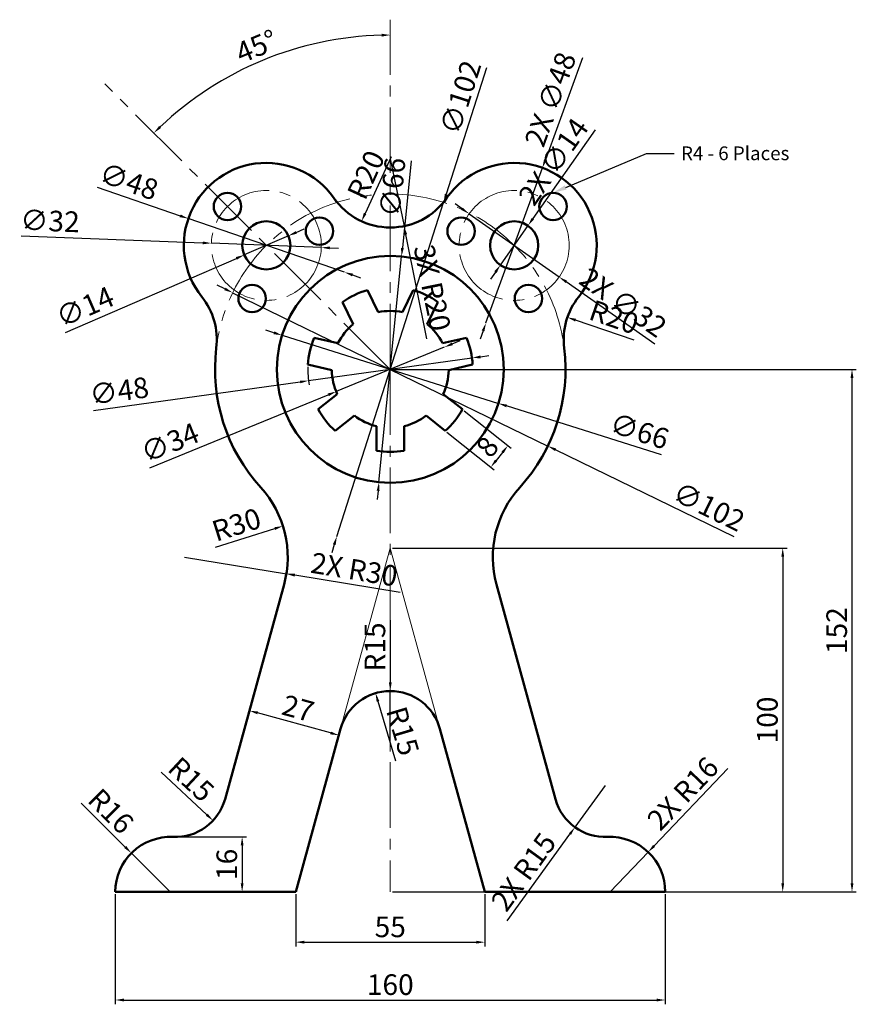
# Model space of a CAD drawing. Units: millimetres. Extents: x 3162 to 3406, y 1893 to 2179.
import ezdxf
from ezdxf import colors
from ezdxf.entities.mleader import LeaderData, LeaderLine
from ezdxf.math import Vec2, Vec3

# ---------------------------------------------------------------- set-up
doc = ezdxf.new("R2010")
doc.units = ezdxf.units.MM
doc.linetypes.add('CENTER2', pattern=[28.575, 19.05, -3.175, 3.175, -3.175])
for name, color, linetype, lineweight in [('M-CNTR', 51, 'CENTER2', 18), ('M-CONS', 8, 'Continuous', 13), ('M-DIMS', 2, 'Continuous', 25), ('M-OUTL', 7, 'Continuous', 50), ('M-TEXT', 7, 'Continuous', 25)]:
    doc.layers.add(name, color=color, linetype=linetype, lineweight=lineweight)
doc.styles.get("Standard").update_dxf_attribs({"font": 'arial.ttf'})
doc.dimstyles.new('ISO-25', dxfattribs={"dimtxt": 6, "dimasz": 2.5, "dimexe": 1.25, "dimexo": 0.625, "dimtad": 1, "dimtxsty": 'Standard', "dimcen": 2.5, "dimadec": 0, "dimazin": 0, "dimtfac": 1, "dimtmove": 0, "dimatfit": 3, "dimfxl": 1, "dimarcsym": 0})

# ---------------------------------------------------------------- blocks, each defined once
blk = doc.blocks.new('*D1')
at = {"layer": 'Defpoints', "color": 0, "transparency": 16777216}
for p in [(3242.62, 1925.58), (3297.62, 1925.58), (3297.62, 1910.95)]:
    blk.add_point(p, dxfattribs=at)
at = {"layer": 'M-DIMS', "color": 0, "lineweight": -2, "transparency": 16777216}
for p, q in [((3242.62, 1924.95), (3242.62, 1909.7)), ((3297.62, 1924.95), (3297.62, 1909.7)), ((3245.12, 1910.95), (3295.12, 1910.95))]:
    blk.add_line(p, q, dxfattribs=at)
at = {"layer": 'M-DIMS', "color": 0, "transparency": 16777216}
for points in [[(3245.12, 1911.37), (3245.12, 1910.53), (3242.62, 1910.95)], [(3295.12, 1911.37), (3295.12, 1910.53), (3297.62, 1910.95)]]:
    blk.add_solid(points, dxfattribs=at)
at = {"layer": 'M-DIMS', "color": 0, "transparency": 16777216, "insert": (3270.12, 1914.63), "char_height": 6, "attachment_point": 5}
blk.add_mtext('55', dxfattribs=at)
blk = doc.blocks.new('*D2')
at = {"layer": 'Defpoints', "color": 0, "transparency": 16777216}
for p in [(3190.12, 1925.58), (3350.12, 1925.58), (3350.12, 1894.13)]:
    blk.add_point(p, dxfattribs=at)
at = {"layer": 'M-DIMS', "color": 0, "lineweight": -2, "transparency": 16777216}
for p, q in [((3190.12, 1924.95), (3190.12, 1892.88)), ((3350.12, 1924.95), (3350.12, 1892.88)), ((3192.62, 1894.13), (3347.62, 1894.13))]:
    blk.add_line(p, q, dxfattribs=at)
at = {"layer": 'M-DIMS', "color": 0, "transparency": 16777216}
for points in [[(3192.62, 1894.54), (3192.62, 1893.71), (3190.12, 1894.13)], [(3347.62, 1894.54), (3347.62, 1893.71), (3350.12, 1894.13)]]:
    blk.add_solid(points, dxfattribs=at)
at = {"layer": 'M-DIMS', "color": 0, "transparency": 16777216, "insert": (3270.12, 1897.82), "char_height": 6, "attachment_point": 5}
blk.add_mtext('160', dxfattribs=at)
blk = doc.blocks.new('*D3')
at = {"layer": 'Defpoints', "color": 0, "transparency": 16777216}
for p in [(3270.12, 2025.58), (3270.12, 1925.58), (3384.31, 1925.58)]:
    blk.add_point(p, dxfattribs=at)
at = {"layer": 'M-DIMS', "color": 0, "lineweight": -2, "transparency": 16777216}
for p, q in [((3270.74, 2025.58), (3385.56, 2025.58)), ((3384.31, 2023.08), (3384.31, 1928.08)), ((3270.74, 1925.58), (3385.56, 1925.58))]:
    blk.add_line(p, q, dxfattribs=at)
at = {"layer": 'M-DIMS', "color": 0, "transparency": 16777216}
for points in [[(3383.9, 2023.08), (3384.73, 2023.08), (3384.31, 2025.58)], [(3383.9, 1928.08), (3384.73, 1928.08), (3384.31, 1925.58)]]:
    blk.add_solid(points, dxfattribs=at)
at = {"layer": 'M-DIMS', "color": 0, "transparency": 16777216, "insert": (3380.62, 1975.58), "char_height": 6, "attachment_point": 5, "rotation": 90}
blk.add_mtext('100', dxfattribs=at)
blk = doc.blocks.new('*D4')
at = {"layer": 'Defpoints', "color": 0, "transparency": 16777216}
for p in [(3270.12, 2077.58), (3404.47, 2077.58), (3270.12, 1925.58)]:
    blk.add_point(p, dxfattribs=at)
at = {"layer": 'M-DIMS', "color": 0, "lineweight": -2, "transparency": 16777216}
for p, q in [((3270.74, 2077.58), (3405.72, 2077.58)), ((3404.47, 1928.08), (3404.47, 2075.08)), ((3270.74, 1925.58), (3405.72, 1925.58))]:
    blk.add_line(p, q, dxfattribs=at)
at = {"layer": 'M-DIMS', "color": 0, "transparency": 16777216}
for points in [[(3404.06, 2075.08), (3404.89, 2075.08), (3404.47, 2077.58)], [(3404.06, 1928.08), (3404.89, 1928.08), (3404.47, 1925.58)]]:
    blk.add_solid(points, dxfattribs=at)
at = {"layer": 'M-DIMS', "color": 0, "transparency": 16777216, "insert": (3400.79, 2001.58), "char_height": 6, "attachment_point": 5, "rotation": 90}
blk.add_mtext('152', dxfattribs=at)
blk = doc.blocks.new('*D5')
at = {"layer": 'Defpoints', "color": 0, "transparency": 16777216}
for p in [(3206.12, 1941.58), (3206.12, 1925.58), (3227.02, 1925.58)]:
    blk.add_point(p, dxfattribs=at)
at = {"layer": 'M-DIMS', "color": 0, "lineweight": -2, "transparency": 16777216}
for p, q in [((3206.74, 1941.58), (3228.27, 1941.58)), ((3227.02, 1939.08), (3227.02, 1928.08)), ((3206.74, 1925.58), (3228.27, 1925.58))]:
    blk.add_line(p, q, dxfattribs=at)
at = {"layer": 'M-DIMS', "color": 0, "transparency": 16777216}
for points in [[(3226.6, 1939.08), (3227.44, 1939.08), (3227.02, 1941.58)], [(3226.6, 1928.08), (3227.44, 1928.08), (3227.02, 1925.58)]]:
    blk.add_solid(points, dxfattribs=at)
at = {"layer": 'M-DIMS', "color": 0, "transparency": 16777216, "insert": (3223.33, 1933.58), "char_height": 6, "attachment_point": 5, "rotation": 90}
blk.add_mtext('16', dxfattribs=at)
blk = doc.blocks.new('*D6')
at = {"layer": 'Defpoints', "color": 0, "transparency": 16777216}
for p in [(3229.62, 1980.15), (3229.12, 1978.3), (3255.66, 1972.99)]:
    blk.add_point(p, dxfattribs=at)
at = {"layer": 'M-DIMS', "color": 0, "lineweight": -2, "transparency": 16777216}
for p, q in [((3229.46, 1979.54), (3228.78, 1977.1)), ((3252.74, 1971.81), (3231.53, 1977.64)), ((3255.49, 1972.38), (3254.82, 1969.94))]:
    blk.add_line(p, q, dxfattribs=at)
at = {"layer": 'M-DIMS', "color": 0, "transparency": 16777216}
for points in [[(3231.64, 1978.04), (3231.42, 1977.24), (3229.12, 1978.3)], [(3252.85, 1972.21), (3252.63, 1971.41), (3255.15, 1971.15)]]:
    blk.add_solid(points, dxfattribs=at)
at = {"layer": 'M-DIMS', "color": 0, "transparency": 16777216, "insert": (3243.1, 1978.23), "char_height": 6, "attachment_point": 5, "rotation": 344.6237}
blk.add_mtext('27', dxfattribs=at)
blk = doc.blocks.new('*D7')
at = {"layer": 'Defpoints', "color": 0, "transparency": 16777216}
for p in [(3194.78, 1936.87), (3206.12, 1925.58)]:
    blk.add_point(p, dxfattribs=at)
at = {"layer": 'M-DIMS', "color": 0, "lineweight": -2, "transparency": 16777216}
for p, q in [((3180.2, 1951.39), (3193.01, 1938.63)), ((3206.12, 1925.58), (3194.78, 1936.87))]:
    blk.add_line(p, q, dxfattribs=at)
at = {"layer": 'M-DIMS', "color": 0, "transparency": 16777216}
blk.add_solid([(3193.3, 1938.93), (3192.72, 1938.34), (3194.78, 1936.87)], dxfattribs=at)
at = {"layer": 'M-DIMS', "color": 0, "transparency": 16777216, "insert": (3188.32, 1948.51), "char_height": 6, "attachment_point": 5, "rotation": 315.1198}
blk.add_mtext('R16', dxfattribs=at)
blk = doc.blocks.new('*D8')
at = {"layer": 'Defpoints', "color": 0, "transparency": 16777216}
for p in [(3207.57, 1956.55), (3218.55, 1946.33)]:
    blk.add_point(p, dxfattribs=at)
at = {"layer": 'M-DIMS', "color": 0, "lineweight": -2, "transparency": 16777216}
blk.add_line((3203.45, 1960.38), (3216.72, 1948.03), dxfattribs=at)
at = {"layer": 'M-DIMS', "color": 0, "transparency": 16777216}
blk.add_solid([(3217.01, 1948.33), (3216.44, 1947.72), (3218.55, 1946.33)], dxfattribs=at)
at = {"layer": 'M-DIMS', "color": 0, "transparency": 16777216, "insert": (3211.69, 1957.76), "char_height": 6, "attachment_point": 5, "rotation": 317.0538}
blk.add_mtext('R15', dxfattribs=at)
blk = doc.blocks.new('*D9')
at = {"layer": 'Defpoints', "color": 0, "transparency": 16777216}
for p in [(3265.84, 1983.39), (3270.12, 1969.01)]:
    blk.add_point(p, dxfattribs=at)
at = {"layer": 'M-DIMS', "color": 0, "lineweight": -2, "transparency": 16777216}
blk.add_line((3271.73, 1963.61), (3266.55, 1980.99), dxfattribs=at)
at = {"layer": 'M-DIMS', "color": 0, "transparency": 16777216}
blk.add_solid([(3266.95, 1981.11), (3266.15, 1980.87), (3265.84, 1983.39)], dxfattribs=at)
at = {"layer": 'M-DIMS', "color": 0, "transparency": 16777216, "insert": (3273.03, 1972.15), "char_height": 6, "attachment_point": 5, "rotation": 286.5756}
blk.add_mtext('R15', dxfattribs=at)
blk = doc.blocks.new('*D10')
at = {"layer": 'Defpoints', "color": 0, "transparency": 16777216}
for p in [(3238.9, 2032), (3210.29, 2022.98)]:
    blk.add_point(p, dxfattribs=at)
at = {"layer": 'M-DIMS', "color": 0, "lineweight": -2, "transparency": 16777216}
blk.add_line((3219.28, 2025.82), (3236.51, 2031.25), dxfattribs=at)
at = {"layer": 'M-DIMS', "color": 0, "transparency": 16777216}
blk.add_solid([(3236.39, 2031.65), (3236.64, 2030.86), (3238.9, 2032)], dxfattribs=at)
at = {"layer": 'M-DIMS', "color": 0, "transparency": 16777216, "insert": (3225.6, 2031.68), "char_height": 6, "attachment_point": 5, "rotation": 17.5099}
blk.add_mtext('R30', dxfattribs=at)
blk = doc.blocks.new('*D11')
at = {"layer": 'Defpoints', "color": 0, "transparency": 16777216}
for p in [(3291.11, 2065.95), (3286.13, 2059.7), (3299.37, 2049.14)]:
    blk.add_point(p, dxfattribs=at)
at = {"layer": 'M-DIMS', "color": 0, "lineweight": -2, "transparency": 16777216}
for p, q in [((3291.6, 2065.56), (3305.33, 2054.61)), ((3286.61, 2059.31), (3300.35, 2048.36)), ((3302.8, 2053.44), (3300.93, 2051.09))]:
    blk.add_line(p, q, dxfattribs=at)
at = {"layer": 'M-DIMS', "color": 0, "transparency": 16777216}
for points in [[(3302.47, 2053.7), (3303.12, 2053.18), (3304.36, 2055.39)], [(3300.6, 2051.35), (3301.25, 2050.83), (3299.37, 2049.14)]]:
    blk.add_solid(points, dxfattribs=at)
at = {"layer": 'M-DIMS', "color": 0, "transparency": 16777216, "insert": (3298.98, 2054.56), "char_height": 6, "attachment_point": 5, "rotation": 51.4286}
blk.add_mtext('8', dxfattribs=at)
blk = doc.blocks.new('*D12')
at = {"layer": 'Defpoints', "color": 0, "transparency": 16777216}
for p in [(3321.67, 2092.7), (3340.59, 2086.22)]:
    blk.add_point(p, dxfattribs=at)
at = {"layer": 'M-DIMS', "color": 0, "lineweight": -2, "transparency": 16777216}
blk.add_line((3341.13, 2086.04), (3324.04, 2091.89), dxfattribs=at)
at = {"layer": 'M-DIMS', "color": 0, "transparency": 16777216}
blk.add_solid([(3324.17, 2092.29), (3323.9, 2091.5), (3321.67, 2092.7)], dxfattribs=at)
at = {"layer": 'M-DIMS', "color": 0, "transparency": 16777216, "insert": (3334.96, 2092.05), "char_height": 6, "attachment_point": 5, "rotation": 341.084}
blk.add_mtext('R20', dxfattribs=at)
blk = doc.blocks.new('*D13')
at = {"layer": 'Defpoints', "color": 0, "transparency": 16777216}
for p in [(3270.12, 2138.85), (3261.77, 2120.68)]:
    blk.add_point(p, dxfattribs=at)
at = {"layer": 'M-DIMS', "color": 0, "lineweight": -2, "transparency": 16777216}
blk.add_line((3270.36, 2139.37), (3262.81, 2122.95), dxfattribs=at)
at = {"layer": 'M-DIMS', "color": 0, "transparency": 16777216}
blk.add_solid([(3262.43, 2123.12), (3263.19, 2122.78), (3261.77, 2120.68)], dxfattribs=at)
at = {"layer": 'M-DIMS', "color": 0, "transparency": 16777216, "insert": (3263.75, 2133.83), "char_height": 6, "attachment_point": 5, "rotation": 65.316}
blk.add_mtext('R20', dxfattribs=at)
blk = doc.blocks.new('*D14')
at = {"layer": 'Defpoints', "color": 0, "transparency": 16777216}
for p in [(3211.35, 2121.43), (3256.76, 2105.85)]:
    blk.add_point(p, dxfattribs=at)
at = {"layer": 'M-DIMS', "color": 0, "lineweight": -2, "transparency": 16777216}
for p, q in [((3184.81, 2130.54), (3208.99, 2122.24)), ((3256.76, 2105.85), (3211.35, 2121.43)), ((3259.12, 2105.04), (3261.49, 2104.23))]:
    blk.add_line(p, q, dxfattribs=at)
at = {"layer": 'M-DIMS', "color": 0, "transparency": 16777216}
for points in [[(3209.13, 2122.63), (3208.85, 2121.85), (3211.35, 2121.43)], [(3259.26, 2105.44), (3258.99, 2104.65), (3256.76, 2105.85)]]:
    blk.add_solid(points, dxfattribs=at)
at = {"layer": 'M-DIMS', "color": 0, "transparency": 16777216, "insert": (3193.81, 2131.52), "char_height": 6, "attachment_point": 5, "rotation": 341.0657}
blk.add_mtext('∅48', dxfattribs=at)
blk = doc.blocks.new('*D15')
at = {"layer": 'Defpoints', "color": 0, "transparency": 16777216}
for p in [(3218.07, 2114.28), (3250.04, 2113.01)]:
    blk.add_point(p, dxfattribs=at)
at = {"layer": 'M-DIMS', "color": 0, "lineweight": -2, "transparency": 16777216}
for p, q in [((3162.77, 2116.47), (3215.57, 2114.38)), ((3250.04, 2113.01), (3218.07, 2114.28)), ((3252.54, 2112.91), (3255.04, 2112.81))]:
    blk.add_line(p, q, dxfattribs=at)
at = {"layer": 'M-DIMS', "color": 0, "transparency": 16777216}
for points in [[(3215.59, 2114.79), (3215.55, 2113.96), (3218.07, 2114.28)], [(3252.56, 2113.32), (3252.52, 2112.49), (3250.04, 2113.01)]]:
    blk.add_solid(points, dxfattribs=at)
at = {"layer": 'M-DIMS', "color": 0, "transparency": 16777216, "insert": (3171.08, 2120), "char_height": 6, "attachment_point": 5, "rotation": 357.726}
blk.add_mtext('∅32', dxfattribs=at)
blk = doc.blocks.new('*D16')
at = {"layer": 'Defpoints', "color": 0, "transparency": 16777216}
for p in [(3240.48, 2116.43), (3227.63, 2110.86)]:
    blk.add_point(p, dxfattribs=at)
at = {"layer": 'M-DIMS', "color": 0, "lineweight": -2, "transparency": 16777216}
for p, q in [((3242.77, 2117.42), (3245.06, 2118.42)), ((3240.48, 2116.43), (3227.63, 2110.86)), ((3175.62, 2088.29), (3225.34, 2109.86))]:
    blk.add_line(p, q, dxfattribs=at)
at = {"layer": 'M-DIMS', "color": 0, "transparency": 16777216}
for points in [[(3242.61, 2117.81), (3242.94, 2117.04), (3240.48, 2116.43)], [(3225.18, 2110.24), (3225.51, 2109.48), (3227.63, 2110.86)]]:
    blk.add_solid(points, dxfattribs=at)
at = {"layer": 'M-DIMS', "color": 0, "transparency": 16777216, "insert": (3181.59, 2095.08), "char_height": 6, "attachment_point": 5, "rotation": 23.4555}
blk.add_mtext('∅14', dxfattribs=at)
blk = doc.blocks.new('*D17')
at = {"layer": 'Defpoints', "color": 0, "transparency": 16777216}
for p in [(3293.89, 2080.88), (3246.35, 2074.28)]:
    blk.add_point(p, dxfattribs=at)
at = {"layer": 'M-DIMS', "color": 0, "lineweight": -2, "transparency": 16777216}
for p, q in [((3293.89, 2080.88), (3246.35, 2074.28)), ((3296.37, 2081.23), (3298.84, 2081.57)), ((3183.75, 2065.58), (3243.87, 2073.93))]:
    blk.add_line(p, q, dxfattribs=at)
blk.add_arc((3270.12, 2077.58), 24, 178.229, 190.8951, dxfattribs=at)
at = {"layer": 'M-DIMS', "color": 0, "transparency": 16777216}
for points in [[(3296.31, 2081.64), (3296.42, 2080.81), (3293.89, 2080.88)], [(3243.81, 2074.34), (3243.93, 2073.52), (3246.35, 2074.28)]]:
    blk.add_solid(points, dxfattribs=at)
at = {"layer": 'M-DIMS', "color": 0, "transparency": 16777216, "insert": (3191.34, 2070.53), "char_height": 6, "attachment_point": 5, "rotation": 7.9109}
blk.add_mtext('∅48', dxfattribs=at)
blk = doc.blocks.new('*D18')
at = {"layer": 'Defpoints', "color": 0, "transparency": 16777216}
for p in [(3285.85, 2084.03), (3254.39, 2071.13)]:
    blk.add_point(p, dxfattribs=at)
at = {"layer": 'M-DIMS', "color": 0, "lineweight": -2, "transparency": 16777216}
for p, q in [((3288.16, 2084.98), (3290.47, 2085.93)), ((3285.85, 2084.03), (3254.39, 2071.13)), ((3200.19, 2048.89), (3252.08, 2070.18))]:
    blk.add_line(p, q, dxfattribs=at)
at = {"layer": 'M-DIMS', "color": 0, "transparency": 16777216}
for points in [[(3288, 2085.37), (3288.32, 2084.6), (3285.85, 2084.03)], [(3251.92, 2070.56), (3252.24, 2069.79), (3254.39, 2071.13)]]:
    blk.add_solid(points, dxfattribs=at)
at = {"layer": 'M-DIMS', "color": 0, "transparency": 16777216, "insert": (3206.29, 2055.56), "char_height": 6, "attachment_point": 5, "rotation": 22.3094}
blk.add_mtext('∅34', dxfattribs=at)
blk = doc.blocks.new('*D19')
at = {"layer": 'Defpoints', "color": 0, "transparency": 16777216}
for p in [(3238.64, 2087.48), (3301.6, 2067.68)]:
    blk.add_point(p, dxfattribs=at)
at = {"layer": 'M-DIMS', "color": 0, "lineweight": -2, "transparency": 16777216}
for p, q in [((3236.25, 2088.23), (3233.87, 2088.98)), ((3238.64, 2087.48), (3301.6, 2067.68)), ((3349.05, 2052.75), (3303.98, 2066.93))]:
    blk.add_line(p, q, dxfattribs=at)
at = {"layer": 'M-DIMS', "color": 0, "transparency": 16777216}
for points in [[(3236.38, 2088.63), (3236.13, 2087.83), (3238.64, 2087.48)], [(3304.11, 2067.33), (3303.86, 2066.53), (3301.6, 2067.68)]]:
    blk.add_solid(points, dxfattribs=at)
at = {"layer": 'M-DIMS', "color": 0, "transparency": 16777216, "insert": (3342.4, 2058.89), "char_height": 6, "attachment_point": 5, "rotation": 342.54}
blk.add_mtext('∅66', dxfattribs=at)
blk = doc.blocks.new('*D20')
at = {"layer": 'Defpoints', "color": 0, "transparency": 16777216}
for p in [(3224.26, 2099.88), (3315.98, 2055.27)]:
    blk.add_point(p, dxfattribs=at)
at = {"layer": 'M-DIMS', "color": 0, "lineweight": -2, "transparency": 16777216}
for p, q in [((3222.01, 2100.98), (3219.76, 2102.07)), ((3224.26, 2099.88), (3315.98, 2055.27)), ((3370.23, 2028.89), (3318.23, 2054.18))]:
    blk.add_line(p, q, dxfattribs=at)
at = {"layer": 'M-DIMS', "color": 0, "transparency": 16777216}
for points in [[(3222.19, 2101.35), (3221.82, 2100.6), (3224.26, 2099.88)], [(3318.41, 2054.55), (3318.05, 2053.81), (3315.98, 2055.27)]]:
    blk.add_solid(points, dxfattribs=at)
at = {"layer": 'M-DIMS', "color": 0, "transparency": 16777216, "insert": (3362.49, 2036.95), "char_height": 6, "attachment_point": 5, "rotation": 334.0641}
blk.add_mtext('∅102', dxfattribs=at)
blk = doc.blocks.new('*D21')
at = {"layer": 'Defpoints', "color": 0, "transparency": 16777216}
for p in [(3270.12, 2179.3), (3244.95, 2171.52), (3187.02, 2160.67), (3270.12, 2077.58), (3270.12, 2077.58)]:
    blk.add_point(p, dxfattribs=at)
at = {"layer": 'M-DIMS', "color": 0, "lineweight": -2, "transparency": 16777216}
blk.add_arc((3270.12, 2077.58), 97.25, 91.4729, 133.5271, dxfattribs=at)
at = {"layer": 'M-DIMS', "color": 0, "transparency": 16777216}
for points in [[(3267.61, 2175.21), (3267.62, 2174.38), (3270.12, 2174.83)], [(3203.43, 2147.79), (3202.85, 2148.39), (3201.35, 2146.35)]]:
    blk.add_solid(points, dxfattribs=at)
at = {"layer": 'M-DIMS', "color": 0, "transparency": 16777216, "insert": (3231.5, 2170.82), "char_height": 6, "attachment_point": 5, "rotation": 22.5}
blk.add_mtext('45°', dxfattribs=at)
blk = doc.blocks.new('MOUNT-PATTERN-D14-3XD8')
for centre, radius in [((-11.31, 11.31), 4), ((0, 0), 7), ((15.45, 4.14), 4), ((-4.14, -15.45), 4)]:
    blk.add_circle(centre, radius)
blk = doc.blocks.new('*D23')
at = {"layer": 'Defpoints', "color": 0, "transparency": 16777216}
for p in [(3285.64, 2126.16), (3254.59, 2029)]:
    blk.add_point(p, dxfattribs=at)
at = {"layer": 'M-DIMS', "color": 0, "lineweight": -2, "transparency": 16777216}
for p, q in [((3298.15, 2165.3), (3286.4, 2128.54)), ((3254.59, 2029), (3285.64, 2126.16)), ((3253.83, 2026.62), (3253.07, 2024.24))]:
    blk.add_line(p, q, dxfattribs=at)
at = {"layer": 'M-DIMS', "color": 0, "transparency": 16777216}
for points in [[(3286.01, 2128.67), (3286.8, 2128.41), (3285.64, 2126.16)], [(3253.44, 2026.74), (3254.23, 2026.49), (3254.59, 2029)]]:
    blk.add_solid(points, dxfattribs=at)
at = {"layer": 'M-DIMS', "color": 0, "transparency": 16777216, "insert": (3291.28, 2156.48), "char_height": 6, "attachment_point": 5, "rotation": 72.2789}
blk.add_mtext('∅102', dxfattribs=at)
blk = doc.blocks.new('*D24')
at = {"layer": 'Defpoints', "color": 0, "transparency": 16777216}
for p in [(3273.4, 2110.42), (3266.84, 2044.74)]:
    blk.add_point(p, dxfattribs=at)
at = {"layer": 'M-DIMS', "color": 0, "lineweight": -2, "transparency": 16777216}
for p, q in [((3276.19, 2138.26), (3273.65, 2112.9)), ((3266.84, 2044.74), (3273.4, 2110.42)), ((3266.59, 2042.26), (3266.34, 2039.77))]:
    blk.add_line(p, q, dxfattribs=at)
at = {"layer": 'M-DIMS', "color": 0, "transparency": 16777216}
for points in [[(3273.24, 2112.94), (3274.06, 2112.86), (3273.4, 2110.42)], [(3266.17, 2042.3), (3267, 2042.21), (3266.84, 2044.74)]]:
    blk.add_solid(points, dxfattribs=at)
at = {"layer": 'M-DIMS', "color": 0, "transparency": 16777216, "insert": (3271.53, 2130.5), "char_height": 6, "attachment_point": 5, "rotation": 84.2904}
blk.add_mtext('∅66', dxfattribs=at)
blk = doc.blocks.new('*D25')
at = {"layer": 'Defpoints', "color": 0, "transparency": 16777216}
for p in [(3210.29, 2022.98), (3239.89, 2018.1)]:
    blk.add_point(p, dxfattribs=at)
at = {"layer": 'M-DIMS', "color": 0, "lineweight": -2, "transparency": 16777216}
for p, q in [((3210.29, 2022.98), (3239.89, 2018.1)), ((3273, 2012.64), (3242.35, 2017.69))]:
    blk.add_line(p, q, dxfattribs=at)
at = {"layer": 'M-DIMS', "color": 0, "transparency": 16777216}
blk.add_solid([(3242.42, 2018.11), (3242.29, 2017.28), (3239.89, 2018.1)], dxfattribs=at)
at = {"layer": 'M-DIMS', "color": 0, "transparency": 16777216, "insert": (3259.51, 2018.61), "char_height": 6, "attachment_point": 5, "rotation": 350.6422}
blk.add_mtext('2X R30', dxfattribs=at)
blk = doc.blocks.new('*D26')
at = {"layer": 'Defpoints', "color": 0, "transparency": 16777216}
for p in [(3314.39, 2136.19), (3297.97, 2091.09)]:
    blk.add_point(p, dxfattribs=at)
at = {"layer": 'M-DIMS', "color": 0, "lineweight": -2, "transparency": 16777216}
for p, q in [((3326.04, 2168.2), (3315.24, 2138.54)), ((3297.97, 2091.09), (3314.39, 2136.19)), ((3297.12, 2088.74), (3296.26, 2086.39))]:
    blk.add_line(p, q, dxfattribs=at)
at = {"layer": 'M-DIMS', "color": 0, "transparency": 16777216}
for points in [[(3314.85, 2138.69), (3315.64, 2138.4), (3314.39, 2136.19)], [(3296.73, 2088.88), (3297.51, 2088.6), (3297.97, 2091.09)]]:
    blk.add_solid(points, dxfattribs=at)
at = {"layer": 'M-DIMS', "color": 0, "transparency": 16777216, "insert": (3317.44, 2155.87), "char_height": 6, "attachment_point": 5, "rotation": 70.0007}
blk.add_mtext('2X ∅48', dxfattribs=at)
blk = doc.blocks.new('*D27')
at = {"layer": 'Defpoints', "color": 0, "transparency": 16777216}
for p in [(3270.12, 2138.85), (3274.12, 2119.25)]:
    blk.add_point(p, dxfattribs=at)
at = {"layer": 'M-DIMS', "color": 0, "lineweight": -2, "transparency": 16777216}
for p, q in [((3270.12, 2138.85), (3274.12, 2119.25)), ((3280.8, 2086.47), (3274.62, 2116.8))]:
    blk.add_line(p, q, dxfattribs=at)
at = {"layer": 'M-DIMS', "color": 0, "transparency": 16777216}
blk.add_solid([(3275.02, 2116.89), (3274.21, 2116.72), (3274.12, 2119.25)], dxfattribs=at)
at = {"layer": 'M-DIMS', "color": 0, "transparency": 16777216, "insert": (3281.58, 2101.15), "char_height": 6, "attachment_point": 5, "rotation": 281.5298}
blk.add_mtext('3X R20', dxfattribs=at)
blk = doc.blocks.new('*D28')
at = {"layer": 'Defpoints', "color": 0, "transparency": 16777216}
for p in [(3293.08, 2122.83), (3319.28, 2104.46)]:
    blk.add_point(p, dxfattribs=at)
at = {"layer": 'M-DIMS', "color": 0, "lineweight": -2, "transparency": 16777216}
for p, q in [((3291.03, 2124.26), (3288.98, 2125.7)), ((3293.08, 2122.83), (3319.28, 2104.46)), ((3347.11, 2084.95), (3321.33, 2103.02))]:
    blk.add_line(p, q, dxfattribs=at)
at = {"layer": 'M-DIMS', "color": 0, "transparency": 16777216}
for points in [[(3291.27, 2124.6), (3290.79, 2123.92), (3293.08, 2122.83)], [(3321.57, 2103.36), (3321.09, 2102.68), (3319.28, 2104.46)]]:
    blk.add_solid(points, dxfattribs=at)
at = {"layer": 'M-DIMS', "color": 0, "transparency": 16777216, "insert": (3337.46, 2096.43), "char_height": 6, "attachment_point": 5, "rotation": 324.9716}
blk.add_mtext('2X ∅32', dxfattribs=at)
blk = doc.blocks.new('*D29')
at = {"layer": 'Defpoints', "color": 0, "transparency": 16777216}
for p in [(3345.16, 1937.16), (3334.12, 1925.58)]:
    blk.add_point(p, dxfattribs=at)
at = {"layer": 'M-DIMS', "color": 0, "lineweight": -2, "transparency": 16777216}
for p, q in [((3368.34, 1961.45), (3346.89, 1938.96)), ((3334.12, 1925.58), (3345.16, 1937.16))]:
    blk.add_line(p, q, dxfattribs=at)
at = {"layer": 'M-DIMS', "color": 0, "transparency": 16777216}
blk.add_solid([(3346.59, 1939.25), (3347.19, 1938.68), (3345.16, 1937.16)], dxfattribs=at)
at = {"layer": 'M-DIMS', "color": 0, "transparency": 16777216, "insert": (3355.81, 1953.66), "char_height": 6, "attachment_point": 5, "rotation": 46.3478}
blk.add_mtext('2X R16', dxfattribs=at)
blk = doc.blocks.new('*D30')
at = {"layer": 'Defpoints', "color": 0, "transparency": 16777216}
for p in [(3332.66, 1956.55), (3323.85, 1944.4)]:
    blk.add_point(p, dxfattribs=at)
at = {"layer": 'M-DIMS', "color": 0, "lineweight": -2, "transparency": 16777216}
for p, q in [((3332.66, 1956.55), (3323.85, 1944.4)), ((3304.11, 1917.19), (3322.38, 1942.38))]:
    blk.add_line(p, q, dxfattribs=at)
at = {"layer": 'M-DIMS', "color": 0, "transparency": 16777216}
blk.add_solid([(3322.05, 1942.63), (3322.72, 1942.14), (3323.85, 1944.4)], dxfattribs=at)
at = {"layer": 'M-DIMS', "color": 0, "transparency": 16777216, "insert": (3309.53, 1930.94), "char_height": 6, "attachment_point": 5, "rotation": 54.0367}
blk.add_mtext('2X R15', dxfattribs=at)
blk = doc.blocks.new('*D31')
at = {"layer": 'Defpoints', "color": 0, "transparency": 16777216}
for p in [(3270.12, 1984.01), (3270.12, 1969.01)]:
    blk.add_point(p, dxfattribs=at)
at = {"layer": 'M-DIMS', "color": 0, "lineweight": -2, "transparency": 16777216}
for p, q in [((3270.12, 2004.64), (3270.12, 1986.51)), ((3270.12, 1969.01), (3270.12, 1984.01))]:
    blk.add_line(p, q, dxfattribs=at)
at = {"layer": 'M-DIMS', "color": 0, "transparency": 16777216}
blk.add_solid([(3269.7, 1986.51), (3270.54, 1986.51), (3270.12, 1984.01)], dxfattribs=at)
at = {"layer": 'M-DIMS', "color": 0, "transparency": 16777216, "insert": (3266.43, 1996.83), "char_height": 6, "attachment_point": 5, "rotation": 89.9981}
blk.add_mtext('R15', dxfattribs=at)
blk = doc.blocks.new('*D32')
at = {"layer": 'Defpoints', "color": 0, "transparency": 16777216}
for p in [(3310.2, 2119.38), (3302.17, 2107.91)]:
    blk.add_point(p, dxfattribs=at)
at = {"layer": 'M-DIMS', "color": 0, "lineweight": -2, "transparency": 16777216}
for p, q in [((3329.71, 2147.25), (3311.63, 2121.42)), ((3302.17, 2107.91), (3310.2, 2119.38)), ((3300.73, 2105.86), (3299.3, 2103.81))]:
    blk.add_line(p, q, dxfattribs=at)
at = {"layer": 'M-DIMS', "color": 0, "transparency": 16777216}
for points in [[(3311.29, 2121.66), (3311.97, 2121.18), (3310.2, 2119.38)], [(3300.39, 2106.1), (3301.07, 2105.62), (3302.17, 2107.91)]]:
    blk.add_solid(points, dxfattribs=at)
at = {"layer": 'M-DIMS', "color": 0, "transparency": 16777216, "insert": (3318.23, 2137.57), "char_height": 6, "attachment_point": 5, "rotation": 55.0009}
blk.add_mtext('2X ∅14', dxfattribs=at)

msp = doc.modelspace()

# ---------------------------------------------------------------- linework, layer by layer
at = {"layer": 'M-CNTR'}
for q in [(3270.119, 2179.296), (3187.024, 2160.674), (3270.119, 1925.579)]:
    msp.add_line((3270.119, 2077.579), q, dxfattribs=at)
for centre in [(3234.056, 2113.642), (3306.181, 2113.642)]:
    msp.add_circle(centre, 16, dxfattribs=at)
msp.add_arc((3270.119, 2077.579), 51, 6.99006, 173.00994, dxfattribs=at)
at = {"layer": 'M-CONS'}
for p, q in [((3255.655, 1972.986), (3270.119, 2025.579)), ((3270.119, 2025.579), (3284.582, 1972.986))]:
    msp.add_line(p, q, dxfattribs=at)
at = {"layer": 'M-OUTL'}
for p, q in [((3266.553, 2094.201), (3263.455, 2100.636)), ((3273.684, 2094.201), (3276.782, 2100.636)), ((3259.346, 2090.73), (3256.247, 2097.165)), ((3280.891, 2090.73), (3283.99, 2097.165)), ((3254.9, 2085.156), (3247.938, 2086.745)), ((3285.337, 2085.156), (3292.299, 2086.745)), ((3253.12, 2077.356), (3246.157, 2078.945)), ((3287.117, 2077.356), (3294.08, 2078.945)), ((3254.707, 2070.405), (3249.123, 2065.952)), ((3285.53, 2070.405), (3291.114, 2065.952)), ((3259.694, 2064.15), (3254.111, 2059.697)), ((3280.543, 2064.15), (3286.126, 2059.697)), ((3266.119, 2061.057), (3266.119, 2053.915)), ((3274.119, 2061.057), (3274.119, 2053.915)), ((3222.038, 1952.568), (3239.213, 2015.024)), ((3301.024, 2015.024), (3318.199, 1952.568)), ((3242.619, 1925.579), (3255.655, 1972.986)), ((3284.582, 1972.986), (3297.619, 1925.579)), ((3242.619, 1925.579), (3190.119, 1925.579)), ((3297.619, 1925.579), (3350.119, 1925.579))]:
    msp.add_line(p, q, dxfattribs=at)
msp.add_circle((3270.119, 2077.579), 33, dxfattribs=at)
for centre, radius, start, end in [((3234.056, 2113.642), 24, 31.39104, 218.55211), ((3306.181, 2113.642), 24, 321.44789, 148.60896), ((3270.119, 2138.851), 20, 214.95512, 325.04488), ((3270.119, 2077.579), 51, 107.65904, 107.78208), ((3270.119, 2077.579), 51, 107.65904, 107.78208), ((3270.119, 2077.579), 51, 72.21792, 72.34096), ((3270.119, 2077.579), 51, 72.21792, 72.34096), ((3270.119, 2077.579), 24, 106.12022, 125.30835), ((3270.119, 2077.579), 24, 54.69165, 73.87978), ((3199.646, 2086.22), 20, 353.00994, 38.55211), ((3340.591, 2086.22), 20, 141.44789, 186.99006), ((3270.119, 2077.579), 17, 77.89467, 102.10533), ((3270.119, 2077.579), 17, 129.32325, 153.5339), ((3270.119, 2077.579), 17, 26.4661, 50.67675), ((3270.119, 2077.579), 24, 157.54879, 176.73693), ((3270.119, 2077.579), 24, 3.26307, 22.45121), ((3270.119, 2077.579), 51, 173.00994, 222.38288), ((3270.119, 2077.579), 51, 317.61712, 6.99006), ((3270.119, 2077.579), 17, 180.75182, 204.96247), ((3270.119, 2077.579), 17, 335.03753, 359.24818), ((3270.119, 2077.579), 24, 208.97736, 228.1655), ((3270.119, 2077.579), 24, 311.8345, 331.02264), ((3270.119, 2077.579), 17, 232.18039, 256.39104), ((3270.119, 2077.579), 17, 283.60896, 307.81961), ((3270.119, 2077.579), 24, 260.40593, 279.59407), ((3210.287, 2022.979), 30, 344.62375, 42.38288), ((3329.95, 2022.979), 30, 137.61712, 195.37625), ((3270.119, 1969.009), 15, 15.37625, 164.62375), ((3207.575, 1956.545), 15, 267.30721, 344.62375), ((3332.662, 1956.545), 15, 195.37625, 272.69279), ((3206.119, 1925.579), 16, 87.30721, 180), ((3334.119, 1925.579), 16, 0, 92.69279)]:
    msp.add_arc(centre, radius, start, end, dxfattribs=at)

# ---------------------------------------------------------------- block references
at = {"layer": 'M-OUTL', "rotation": 150.0000000000003}
msp.add_blockref('MOUNT-PATTERN-D14-3XD8', (3306.181, 2113.642), dxfattribs=at)
at = {"layer": 'M-OUTL'}
msp.add_blockref('MOUNT-PATTERN-D14-3XD8', (3234.056, 2113.642), dxfattribs=at)

# ---------------------------------------------------------------- dimensions: what is measured, and where the dimension line sits
at = {"layer": 'M-DIMS'}
dim = msp.add_angular_dim_2l(base=(3244.948, 2171.516), line1=((3270.119, 2077.579), (3187.024, 2160.674)), line2=((3270.119, 2077.579), (3270.119, 2179.296)), dimstyle='ISO-25', override={"dimclrd": 0, "dimclre": 0, "dimclrt": 0}, dxfattribs=at)
dim.commit()
dim.dimension.update_dxf_attribs({"geometry": '*D21', "text_midpoint": (3231.496, 2170.823)})
for p1, p2, picture, middle in [((3297.973, 2091.089), (3314.389, 2136.194), '*D26', (3321.069, 2154.547)), ((3293.079, 2122.825), (3319.283, 2104.458), '*D28', (3335.245, 2093.269))]:
    dim = msp.add_diameter_dim_2p(p1=p1, p2=p2, text='2X <>', dimstyle='ISO-25', override={"dimdec": 0, "dimlfac": 1, "dimrnd": 0, "dimzin": 0, "dimdsep": 46, "dimlunit": 2}, dxfattribs=at)
    dim.commit()
    dim.dimension.update_dxf_attribs({"geometry": picture, "text_midpoint": middle, "dimtype": 163})
for p1, p2, override, picture, middle in [((3254.595, 2028.999), (3285.642, 2126.159), {"dimdec": 0, "dimlfac": 1, "dimrnd": 0, "dimzin": 0, "dimdsep": 46, "dimlunit": 2}, '*D23', (3294.956, 2155.307)), ((3256.757, 2105.854), (3211.355, 2121.429), {"dimclrd": 0, "dimclre": 0, "dimclrt": 0}, '*D14', (3192.559, 2127.877)), ((3266.835, 2044.743), (3273.402, 2110.416), {"dimdec": 0, "dimlfac": 1, "dimrnd": 0, "dimzin": 0, "dimdsep": 46, "dimlunit": 2}, '*D24', (3275.371, 2130.117)), ((3250.043, 2113.007), (3218.069, 2114.277), {"dimclrd": 0, "dimclre": 0, "dimclrt": 0}, '*D15', (3170.924, 2116.149)), ((3240.478, 2116.428), (3227.634, 2110.855), {"dimclrd": 0, "dimclre": 0, "dimclrt": 0}, '*D16', (3183.123, 2091.542)), ((3224.255, 2099.885), (3315.982, 2055.274), {"dimclrd": 0, "dimclre": 0, "dimclrt": 0}, '*D20', (3360.799, 2033.477)), ((3238.639, 2087.481), (3301.598, 2067.678), {"dimclrd": 0, "dimclre": 0, "dimclrt": 0}, '*D19', (3341.245, 2055.208)), ((3285.846, 2084.033), (3254.391, 2071.126), {"dimclrd": 0, "dimclre": 0, "dimclrt": 0}, '*D18', (3207.75, 2051.988)), ((3293.89, 2080.882), (3246.347, 2074.276), {"dimclrd": 0, "dimclre": 0, "dimclrt": 0}, '*D17', (3191.869, 2066.706))]:
    dim = msp.add_diameter_dim_2p(p1=p1, p2=p2, dimstyle='ISO-25', override=override, dxfattribs=at)
    dim.commit()
    dim.dimension.update_dxf_attribs({"geometry": picture, "text_midpoint": middle, "dimtype": 163})
dim = msp.add_diameter_dim_2p(p1=(3302.166, 2107.908), p2=(3310.196, 2119.376), text='2X <>', dimstyle='ISO-25', override={"dimdec": 0, "dimlfac": 1, "dimrnd": 0, "dimzin": 0, "dimdsep": 46, "dimlunit": 2}, dxfattribs=at)
dim.commit()
dim.dimension.update_dxf_attribs({"geometry": '*D32', "text_midpoint": (3321.387, 2135.359)})
for center, mpoint, picture, middle in [((3270.119, 2138.851), (3261.766, 2120.678), '*D13', (3267.105, 2132.294)), ((3340.591, 2086.22), (3321.671, 2092.703), '*D12', (3333.764, 2088.559)), ((3210.287, 2022.979), (3238.897, 2032.005), '*D10', (3226.706, 2028.159)), ((3270.119, 1969.009), (3265.839, 1983.386), '*D9', (3269.495, 1971.102)), ((3207.575, 1956.545), (3218.555, 1946.325), '*D8', (3209.174, 1955.057))]:
    dim = msp.add_radius_dim(center=center, mpoint=mpoint, dimstyle='ISO-25', override={"dimclrd": 0, "dimclre": 0, "dimclrt": 0}, dxfattribs=at)
    dim.commit()
    dim.dimension.update_dxf_attribs({"geometry": picture, "text_midpoint": middle, "dimtype": 164})
for center, mpoint, text, picture, middle in [((3270.119, 2138.851), (3274.116, 2119.254), '3X <>', '*D27', (3281.575, 2101.153)), ((3210.287, 2022.979), (3239.888, 2018.101), '2X <>', '*D25', (3259.512, 2018.607)), ((3334.119, 1925.579), (3345.163, 1937.156), '2X <>', '*D29', (3355.809, 1953.658)), ((3332.662, 1956.545), (3323.853, 1944.404), '2X <>', '*D30', (3309.526, 1930.938))]:
    dim = msp.add_radius_dim(center=center, mpoint=mpoint, text=text, dimstyle='ISO-25', override={"dimdec": 0, "dimlfac": 1, "dimrnd": 0, "dimzin": 0, "dimdsep": 46, "dimlunit": 2}, dxfattribs=at)
    dim.commit()
    dim.dimension.update_dxf_attribs({"geometry": picture, "text_midpoint": middle})
for base, p1, p2, picture, middle in [((3404.474, 2077.579), (3270.119, 1925.579), (3270.119, 2077.579), '*D4', (3400.785, 2001.579)), ((3384.313, 1925.579), (3270.119, 2025.579), (3270.119, 1925.579), '*D3', (3380.625, 1975.579)), ((3227.02, 1925.579), (3206.119, 1941.579), (3206.119, 1925.579), '*D5', (3223.331, 1933.579))]:
    dim = msp.add_linear_dim(base=base, p1=p1, p2=p2, angle=90, dimstyle='ISO-25', override={"dimclrd": 0, "dimclre": 0, "dimclrt": 0}, dxfattribs=at)
    dim.commit()
    dim.dimension.update_dxf_attribs({"geometry": picture, "text_midpoint": middle})
for p1, p2, distance, picture, middle in [((3291.114, 2065.952), (3286.126, 2059.697), 16.939, '*D11', (3298.98, 2054.563)), ((3255.655, 1972.986), (3229.622, 1980.145), 1.909, '*D6', (3243.097, 1978.232))]:
    dim = msp.add_aligned_dim(p1=p1, p2=p2, distance=distance, dimstyle='ISO-25', override={"dimclrd": 0, "dimclre": 0, "dimclrt": 0}, dxfattribs=at)
    dim.commit()
    dim.dimension.update_dxf_attribs({"geometry": picture, "text_midpoint": middle})
for center, mpoint, override, picture, middle in [((3270.119, 1969.009), (3270.119, 1984.009), {"dimdec": 0, "dimlfac": 1, "dimrnd": 0, "dimzin": 0, "dimdsep": 46, "dimlunit": 2}, '*D31', (3266.431, 1996.825)), ((3206.119, 1925.579), (3194.781, 1936.869), {"dimclrd": 0, "dimclre": 0, "dimclrt": 0}, '*D7', (3188.32, 1948.509))]:
    dim = msp.add_radius_dim(center=center, mpoint=mpoint, dimstyle='ISO-25', override=override, dxfattribs=at)
    dim.commit()
    dim.dimension.update_dxf_attribs({"geometry": picture, "text_midpoint": middle})
for base, p1, p2, picture, middle in [((3350.119, 1894.127), (3190.119, 1925.579), (3350.119, 1925.579), '*D2', (3270.119, 1897.816)), ((3297.619, 1910.951), (3242.619, 1925.579), (3297.619, 1925.579), '*D1', (3270.119, 1914.628))]:
    dim = msp.add_linear_dim(base=base, p1=p1, p2=p2, dimstyle='ISO-25', override={"dimclrd": 0, "dimclre": 0, "dimclrt": 0}, dxfattribs=at)
    dim.commit()
    dim.dimension.update_dxf_attribs({"geometry": picture, "text_midpoint": middle})

# ---------------------------------------------------------------- leaders
at = {"layer": 'M-TEXT'}
ml = msp.add_multileader_mtext('Standard', dxfattribs=at)
ml.set_content('R4 - 6 Places', color=256)
ml.set_leader_properties()
ml.build(insert=Vec2(0, 0))
ctx = ml.context
ctx.base_point, ctx.plane_origin = Vec3(3352.721, 2140.397), Vec3(3317.495, 2128.955)
notes = []
notes.append((ctx, [(0, (1, 1, 0), (3344.721, 2140.397), (1, 0), 8, [(0, [(3317.495, 2128.955)], 0, [])])]))
ctx.mtext.insert, ctx.mtext.flow_direction = Vec3(3354.721, 2142.431), 5
for ctx, leaders in notes:
    for number, flags, end, landing, length, lines in leaders:
        leader = LeaderData()
        leader.index, (leader.has_last_leader_line, leader.has_dogleg_vector, leader.attachment_direction) = number, flags
        leader.last_leader_point, leader.dogleg_vector, leader.dogleg_length = Vec3(end), Vec3(landing), length
        for number, points, colour, breaks in lines:
            line = LeaderLine()
            line.index, line.vertices, line.color, line.breaks = number, Vec3.list(points), colors.encode_raw_color(colour), breaks
            leader.lines.append(line)
        ctx.leaders.append(leader)

doc.saveas('drawing.dxf')
